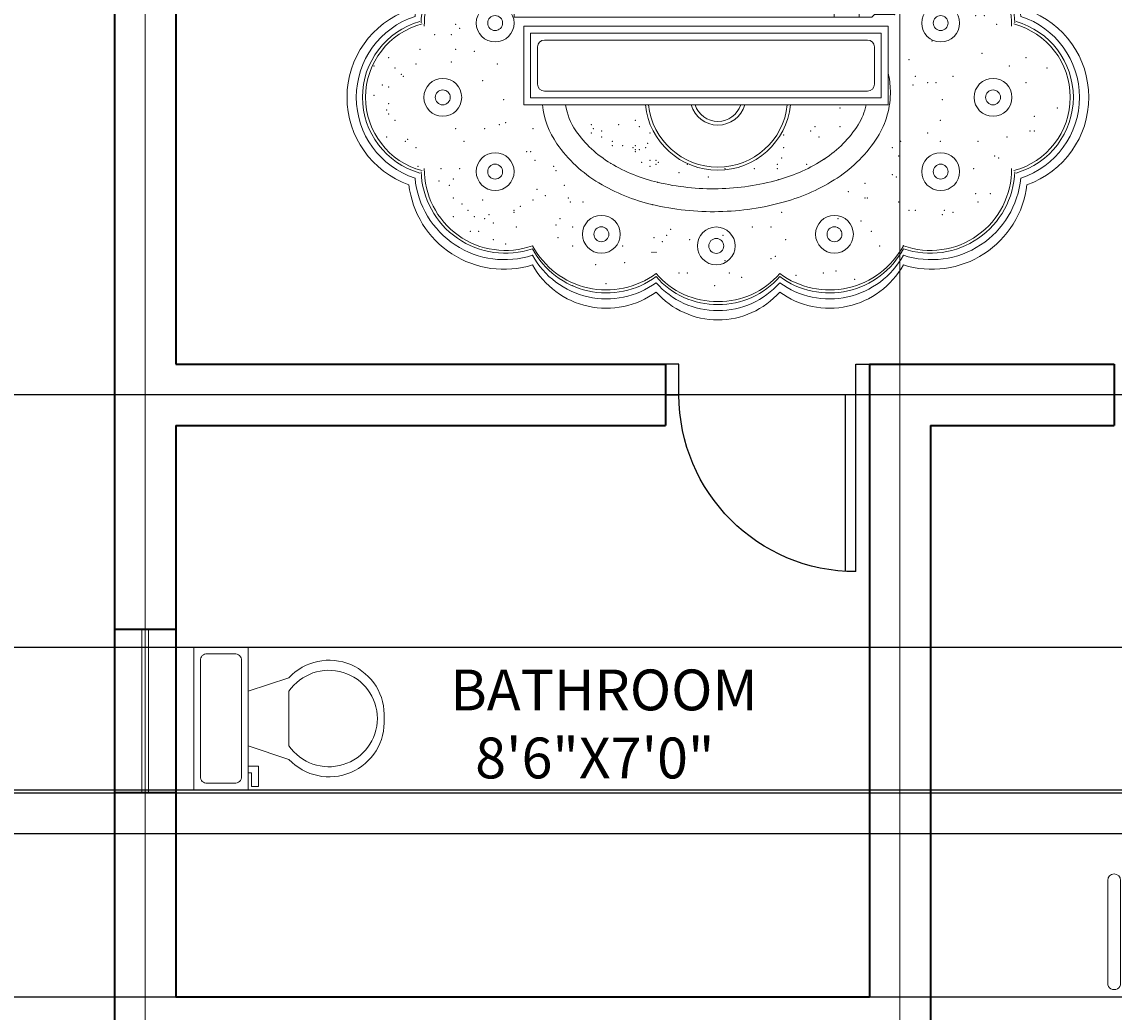
# Model space of a CAD drawing. Units: inches. Extents: x 5716 to 6907, y 12769 to 13594.
# Tile 13 of 17: x 6254 to 6414, y 13204 to 13349. Entities that reach past the tile are written whole.
import ezdxf

# ---------------------------------------------------------------- set-up
doc = ezdxf.new("R2010")
doc.units = ezdxf.units.IN
for name, color, linetype, lineweight in [('A-ANNO-DIMS', 2, 'Continuous', 18), ('A-AREA-IDEN', 7, 'Continuous', 18), ('A-DOOR', 4, 'Continuous', 25), ('A-FLOR-FIXT', 9, 'Continuous', 18), ('A-FURN', 8, 'Continuous', 18), ('A-GLAZ', 4, 'Continuous', 18), ('A-GRID', 8, 'Continuous', 13), ('A-WALL', 7, 'Continuous', 35)]:
    doc.layers.add(name, color=color, linetype=linetype, lineweight=lineweight)
doc.styles.get("Standard").update_dxf_attribs({"font": 'arial.ttf'})
doc.dimstyles.get("Standard").update_dxf_attribs({"dimtxt": 0.18, "dimasz": 0.18, "dimexe": 0.18, "dimexo": 0.0625, "dimgap": 0.09, "dimtad": 0, "dimtih": 1, "dimtoh": 1, "dimdec": 4, "dimzin": 0, "dimdsep": 46, "dimtxsty": 'Standard', "dimcen": 0.09, "dimadec": 0, "dimazin": 0, "dimtfac": 1, "dimtdec": 4, "dimtofl": 0, "dimtmove": 0, "dimatfit": 3, "dimfxl": 1, "dimtolj": 1, "dimtzin": 0, "dimarcsym": 0})

# ---------------------------------------------------------------- blocks, each defined once
blk = doc.blocks.new('A$C1EC128A1')
for p, q in [((0.1147, 3.56), (3.0187, 3.56)), ((0.1147, 3.555), (0.1147, 3.511)), ((3.0187, 3.555), (3.0187, 3.511)), ((0.1147, 3.511), (3.0187, 3.511)), ((0.2027, 3.511), (0.2027, 3.4616)), ((0.6977, 3.511), (0.6977, 3.016)), ((0.7417, 3.511), (0.7417, 2.972)), ((0.7857, 3.4835), (1.5392, 3.4835)), ((0.7857, 3.4835), (0.7857, 3.126)), ((1.5392, 3.126), (1.5392, 3.4835)), ((1.5942, 3.126), (1.5942, 3.4835)), ((1.5942, 3.4835), (2.3477, 3.4835)), ((2.3477, 3.4835), (2.3477, 3.126)), ((2.3917, 3.511), (2.3917, 3.1535)), ((2.4357, 3.511), (2.4357, 3.016)), ((2.9307, 3.511), (2.9307, 3.016)), ((0.2027, 3.4601), (0.2027, 3.016)), ((0.3741, 3.1815), (0.5297, 3.337)), ((0.3741, 3.337), (0.5297, 3.1815)), ((2.6038, 3.337), (2.7594, 3.1815)), ((2.7594, 3.337), (2.6038, 3.1815)), ((1.5392, 3.1535), (1.5942, 3.1535)), ((2.3477, 3.1535), (2.4027, 3.1535)), ((2.4027, 3.1535), (2.4027, 1.432)), ((0.7307, 2.961), (0.8957, 3.126)), ((0.7857, 3.126), (1.5392, 3.126)), ((0.9507, 3.126), (0.9507, 2.9335)), ((1.0607, 3.126), (1.0607, 2.8235)), ((1.5942, 3.126), (2.3477, 3.126)), ((0.2027, 3.016), (0.6977, 3.016)), ((1.0607, 3.0435), (2.4027, 3.0435)), ((2.9307, 3.016), (2.4357, 3.016)), ((0.7307, 2.961), (0.7307, 1.322)), ((0.7307, 2.9335), (0.9507, 2.9335)), ((0.7307, 2.8235), (1.0607, 2.8235)), ((2.1277, 1.597), (2.4027, 1.597)), ((2.1277, 1.597), (2.1277, 1.322)), ((2.2377, 1.487), (2.2377, 1.322)), ((2.2377, 1.487), (2.4027, 1.487)), ((2.2927, 1.322), (2.4027, 1.432)), ((2.3917, 1.421), (2.3917, 1.333)), ((0.7307, 1.322), (2.2927, 1.322)), ((2.3037, 1.333), (2.3917, 1.333)), ((0.7721, 1.282), (2.3633, 1.282)), ((0.7721, 0.939), (0.7721, 1.282)), ((0.8021, 1.252), (2.3333, 1.252)), ((0.8021, 0.969), (0.8021, 1.252)), ((2.3333, 1.252), (2.3333, 0.969)), ((2.3633, 1.282), (2.3633, 0.939)), ((0.8621, 1.222), (2.2733, 1.222)), ((0.8321, 1.029), (0.8321, 1.192)), ((2.3033, 1.192), (2.3033, 1.029)), ((2.3333, 0.969), (0.8021, 0.969)), ((2.2733, 0.999), (0.8621, 0.999)), ((2.3633, 0.939), (0.7721, 0.939))]:
    blk.add_line(p, q)
for centre, radius in [((0.4519, 3.2593), 0.22), ((2.6816, 3.2593), 0.22), ((0.4519, 3.2593), 0.11), ((2.6816, 3.2593), 0.11), ((0.647, 1.2961), 0.0826), ((2.593, 1.2961), 0.0826), ((0.647, 1.2961), 0.0326), ((2.593, 1.2961), 0.0326), ((0.4183, 0.9718), 0.0826), ((2.8217, 0.9718), 0.0826), ((0.4183, 0.9718), 0.0326), ((2.8217, 0.9718), 0.0326), ((0.647, 0.6475), 0.0826), ((2.593, 0.6475), 0.0826), ((0.647, 0.6475), 0.0326), ((2.593, 0.6475), 0.0326), ((1.1109, 0.3741), 0.0826), ((2.1291, 0.3741), 0.0826), ((1.1109, 0.3741), 0.0326), ((1.6128, 0.3232), 0.0826), ((2.1291, 0.3741), 0.0326), ((1.6128, 0.3232), 0.0326)]:
    blk.add_circle(centre, radius)
for centre, radius, start, end in [((0.6854, 1.3045), 0.4183, 83.7824, 173.2515), ((2.5546, 1.3045), 0.4183, 6.7485, 111.2795), ((0.6884, 1.2877), 0.3932, 83.8157, 174.53), ((2.5516, 1.2877), 0.3932, 5.47, 112.249), ((0.6921, 1.2838), 0.369, 83.9971, 177.9976), ((0.6913, 1.2866), 0.3539, 83.6051, 180.6699), ((2.5479, 1.2838), 0.369, 2.0024, 113.1536), ((2.5487, 1.2866), 0.3539, 359.3301, 114.3551), ((0.4048, 0.972), 0.4048, 109.4527, 180), ((2.8352, 0.972), 0.4048, 0, 70.5473), ((0.4119, 0.972), 0.3714, 108.0256, 180), ((0.411, 0.972), 0.3435, 105.7891, 180), ((0.4122, 0.972), 0.3312, 104.766, 180), ((2.8278, 0.972), 0.3312, 0, 75.234), ((2.829, 0.972), 0.3435, 0, 74.2109), ((2.8281, 0.972), 0.3714, 0, 71.9744), ((0.8621, 1.192), 0.03, 90, 180), ((2.2733, 1.192), 0.03, 0, 90), ((2.0084, 0.9935), 0.365, 1.1782, 13.4812), ((0.8621, 1.029), 0.03, 180, 270), ((2.2733, 1.029), 0.03, 270, 0), ((0.4048, 0.972), 0.4048, 180, 250.5473), ((0.4119, 0.972), 0.3714, 180, 251.9744), ((0.411, 0.972), 0.3435, 180, 254.2109), ((0.4122, 0.972), 0.3312, 180, 255.234), ((2.0084, 0.9935), 0.365, 327.6239, 1.1782), ((2.8278, 0.972), 0.3312, 284.766, 0), ((2.829, 0.972), 0.3435, 285.7891, 0), ((2.8281, 0.972), 0.3714, 288.0256, 0), ((2.8352, 0.972), 0.4048, 289.4527, 0), ((1.2169, 0.9773), 0.365, 186.0197, 214.7326), ((1.2169, 0.9773), 0.265, 188.3055, 214.7326), ((1.62, 0.972), 0.3185, 185.9507, 354.0493), ((1.62, 0.972), 0.305, 186.2151, 353.7849), ((1.62, 0.972), 0.1215, 195.7695, 344.2305), ((1.62, 0.972), 0.105, 198.3291, 341.6709), ((2.0084, 0.9935), 0.265, 327.6239, 348.1186), ((1.4035, 1.1066), 0.492, 214.7326, 239.1926), ((1.8167, 1.1151), 0.492, 303.1639, 327.6239), ((1.4035, 1.1066), 0.592, 214.7326, 239.1926), ((1.8167, 1.1151), 0.592, 303.1639, 327.6239), ((1.5241, 1.3089), 0.7275, 239.1926, 256.6746), ((1.6878, 1.3123), 0.7275, 285.6819, 303.1639), ((0.6921, 0.6602), 0.369, 182.0024, 288.623), ((0.6913, 0.6574), 0.3539, 179.3301, 289.5945), ((2.5487, 0.6574), 0.3539, 250.4055, 0.6699), ((2.5479, 0.6602), 0.369, 251.377, 357.9976), ((0.6854, 0.6395), 0.4183, 186.7485, 287.3233), ((0.6884, 0.6563), 0.3932, 185.47, 288.0175), ((1.5241, 1.3089), 0.8275, 239.1926, 256.6746), ((1.5995, 1.627), 1.0544, 256.6746, 271.1782), ((1.5995, 1.627), 1.0544, 271.1782, 285.6819), ((1.6878, 1.3123), 0.8275, 285.6819, 303.1639), ((2.5516, 0.6563), 0.3932, 251.9825, 354.53), ((2.5546, 0.6395), 0.4183, 252.6767, 353.2515), ((1.5995, 1.627), 1.1544, 256.6746, 271.1782), ((1.5995, 1.627), 1.1544, 271.1782, 285.6819), ((1.1328, 0.4977), 0.3665, 208.2914, 306.3479), ((1.1328, 0.4842), 0.3665, 208.2914, 306.3479), ((2.1072, 0.4977), 0.3665, 233.6521, 331.7086), ((2.1072, 0.4842), 0.3665, 233.6521, 331.7086), ((1.133, 0.4609), 0.369, 208.9302, 306.0262), ((1.1324, 0.4204), 0.3694, 209.2201, 306.079), ((2.107, 0.4609), 0.369, 233.9738, 331.0698), ((2.1076, 0.4204), 0.3694, 233.921, 330.7799), ((1.6145, 0.4295), 0.3486, 220.6393, 270.9052), ((1.6255, 0.4295), 0.3486, 269.0948, 319.3607), ((1.6145, 0.416), 0.3486, 220.6393, 270.9052), ((1.62, 0.4004), 0.3599, 221.3878, 270), ((1.6255, 0.416), 0.3486, 269.0948, 319.3607), ((1.62, 0.4004), 0.3599, 270, 318.6122), ((1.62, 0.36), 0.36, 221.4185, 270), ((1.62, 0.36), 0.36, 270, 318.5815)]:
    blk.add_arc(centre, radius, start, end)
for p in [(0.5654, 1.5652), (0.6657, 1.5561), (2.4819, 1.5378), (2.5184, 1.5744), (2.5366, 1.5378), (2.6097, 1.5378), (2.71, 1.5561), (0.4376, 1.5104), (0.5471, 1.5013), (0.5471, 1.4922), (0.6475, 1.5013), (0.465, 1.4739), (2.6735, 1.4739), (2.6735, 1.4556), (2.7648, 1.4465), (0.4285, 1.4282), (0.4285, 1.3917), (0.5562, 1.3917), (0.5927, 1.3917), (0.6566, 1.41), (2.6005, 1.4191), (2.8013, 1.4191), (0.4011, 1.3552), (0.4285, 1.3734), (2.7648, 1.346), (0.4741, 1.2912), (2.3917, 1.333), (2.7465, 1.3278), (2.7831, 1.3278), (2.8378, 1.2912), (0.3828, 1.2456), (0.4558, 1.2456), (0.4923, 1.273), (2.5549, 1.2182), (0.1821, 1.1451), (0.3189, 1.1816), (0.4741, 1.1816), (0.5562, 1.1725), (2.7739, 1.1634), (2.9656, 1.1451), (0.1182, 1.1085), (0.2094, 1.0994), (0.3007, 1.1177), (0.4558, 1.1268), (0.6566, 1.1177), (2.4545, 1.1359), (2.8926, 1.1085), (3.0568, 1.0994), (0.2368, 1.072), (0.2459, 1.0629), (2.4819, 1.0629), (2.6462, 1.0629), (0.1547, 1.0263), (0.1821, 1.0172), (0.5927, 1.0446), (2.4728, 1.0263), (2.5366, 1.0355), (2.5731, 1.0355), (2.9656, 1.0355), (0.1182, 0.9807), (0.684, 0.9624), (2.6005, 0.9624), (0.1729, 0.9167), (0.1821, 0.9441), (1.3032, 0.939), (1.3168, 0.939), (2.1533, 0.9259), (3.1025, 0.9259), (0.1821, 0.8985), (0.2094, 0.8711), (0.6931, 0.8619), (1.259, 0.8711), (2.5914, 0.8711), (3.0021, 0.8893), (0.4741, 0.8345), (0.6019, 0.8345), (0.6657, 0.8528), (0.8118, 0.8345), (0.9992, 0.8263), (1.0673, 0.8528), (1.0673, 0.8163), (1.0764, 0.8345), (1.1129, 0.8254), (1.1859, 0.8528), (1.2772, 0.8437), (1.3228, 0.8163), (2.0256, 0.8254), (2.0438, 0.8437), (2.0438, 0.8437), (2.1533, 0.8437), (2.5366, 0.8163), (2.9838, 0.8254), (3.0021, 0.8254), (0.1729, 0.798), (0.2551, 0.7797), (0.2642, 0.7889), (0.5106, 0.7797), (1.1129, 0.798), (1.1586, 0.7797), (1.3137, 0.7706), (1.9069, 0.8071), (2.0621, 0.798), (2.418, 0.7797), (2.5914, 0.7797), (2.7557, 0.7797), (2.8834, 0.798), (0.3007, 0.7523), (0.7844, 0.7341), (0.8026, 0.7341), (1.1586, 0.7615), (1.2042, 0.7615), (1.2498, 0.7523), (1.259, 0.7615), (1.259, 0.7432), (1.259, 0.7341), (1.2772, 0.7432), (1.3046, 0.7523), (1.9069, 0.7523), (2.3815, 0.7523), (2.4089, 0.7158), (2.8287, 0.7158), (0.3098, 0.6701), (0.8209, 0.6975), (0.903, 0.6701), (1.1515, 0.684), (1.1515, 0.684), (1.1515, 0.684), (1.2863, 0.6884), (1.3228, 0.6975), (1.3228, 0.6701), (1.3502, 0.6975), (1.3502, 0.6793), (1.3593, 0.6884), (1.4871, 0.6793), (1.8795, 0.6793), (1.8978, 0.7067), (2.0073, 0.6793), (2.0858, 0.7033), (2.8469, 0.7067), (0.4102, 0.661), (0.4923, 0.661), (0.9122, 0.6519), (1.4506, 0.6427), (1.5784, 0.6245), (1.6514, 0.661), (1.6514, 0.661), (1.7792, 0.661), (1.8795, 0.661), (2.3815, 0.6336), (2.3997, 0.6245), (2.7374, 0.661), (0.4011, 0.6062), (0.4467, 0.5879), (0.465, 0.6153), (0.9487, 0.5879), (1.3564, 0.601), (1.8845, 0.6118), (2.2629, 0.597), (0.465, 0.5331), (0.83, 0.5696), (0.8665, 0.5422), (0.9669, 0.5331), (2.1898, 0.5605), (2.2629, 0.5331), (2.272, 0.5331), (2.7465, 0.5514), (2.8104, 0.5514), (0.5015, 0.5057), (0.5289, 0.4783), (0.5927, 0.524), (0.7296, 0.4783), (0.757, 0.4966), (0.8118, 0.524), (0.976, 0.5148), (1.0308, 0.5148), (1.3334, 0.5037), (2.4089, 0.5148), (2.4545, 0.4783), (2.4819, 0.4783), (2.6097, 0.4783), (2.7557, 0.5148), (0.465, 0.4509), (0.5562, 0.4509), (0.6019, 0.4418), (0.6201, 0.46), (0.7296, 0.4692), (0.9304, 0.4418), (1.8978, 0.4692), (2.1442, 0.4418), (2.2446, 0.4326), (2.6005, 0.46), (2.6462, 0.4692), (0.538, 0.387), (0.5745, 0.387), (0.6384, 0.4235), (0.7388, 0.4052), (0.7388, 0.4052), (0.9122, 0.4144), (0.9852, 0.4052), (1.4141, 0.3961), (1.77, 0.4052), (1.8522, 0.4052), (2.2902, 0.387), (0.6384, 0.3504), (0.9213, 0.3596), (1.3411, 0.3596), (1.3776, 0.3413), (1.3959, 0.3687), (1.4962, 0.3504), (1.6423, 0.3687), (1.9161, 0.3504), (0.6931, 0.3322), (0.9852, 0.323), (1.2042, 0.323), (1.332, 0.2956), (1.3411, 0.2956), (1.3502, 0.2956), (2.3267, 0.323), (2.43, 0.324), (0.81, 0.2824), (1.0856, 0.2408), (1.2133, 0.25), (1.6514, 0.2591), (1.8522, 0.2682), (1.8704, 0.2774), (1.35, 0.2025), (1.4506, 0.2043), (1.4871, 0.2043), (1.6696, 0.2043), (1.9617, 0.1952), (2.0803, 0.2043), (2.1351, 0.2134), (0.9852, 0.1495), (1.1312, 0.1586), (1.6058, 0.1495), (1.7244, 0.186), (2.2172, 0.1769)]:
    blk.add_point(p)
blk = doc.blocks.new('A$C405465A0')
for p, q in [((1.1305, 2.1034), (1.5301, 2.1034)), ((1.5301, 2.0534), (1.1305, 2.0534)), ((1.1304, 1.6481), (1.1055, 2.0017)), ((1.279, 2.0284), (1.1105, 1.9312)), ((1.4665, 2.0284), (1.1178, 1.8271)), ((1.1305, 2.0284), (1.5301, 2.0284)), ((1.1428, 1.625), (1.1428, 2.0284)), ((1.5427, 1.8271), (1.1941, 2.0284)), ((1.2365, 1.625), (1.2365, 2.0284)), ((1.3303, 1.625), (1.3303, 2.0284)), ((1.5501, 1.9312), (1.3816, 2.0284)), ((1.424, 1.625), (1.424, 2.0284)), ((1.5178, 1.625), (1.5178, 2.0284)), ((1.555, 2.0017), (1.5301, 1.6481)), ((1.5354, 1.7231), (1.1078, 1.97)), ((1.5528, 1.97), (1.1252, 1.7231)), ((0.9452, 1.8803), (0.5455, 1.8803)), ((2.1342, 1.8803), (1.7345, 1.8803)), ((0.5455, 1.8303), (0.9452, 1.8303)), ((1.5178, 1.625), (1.1157, 1.8572)), ((1.5449, 1.8572), (1.1428, 1.625)), ((1.7345, 1.8303), (2.1342, 1.8303)), ((0.5268, 1.6904), (0.7259, 1.8053)), ((0.9452, 1.8053), (0.5455, 1.8053)), ((0.5578, 1.6), (0.5578, 1.8053)), ((0.5578, 1.6), (0.9134, 1.8053)), ((0.5773, 1.8053), (0.9328, 1.6)), ((0.6516, 1.6), (0.6516, 1.8053)), ((0.7453, 1.6), (0.7453, 1.8053)), ((0.7648, 1.8053), (0.9639, 1.6904)), ((0.8391, 1.6), (0.8391, 1.8053)), ((0.9328, 1.6), (0.9328, 1.8053)), ((1.7158, 1.6904), (1.9149, 1.8053)), ((2.1342, 1.8053), (1.7345, 1.8053)), ((1.7468, 1.6), (1.7468, 1.8053)), ((1.7468, 1.6), (2.1024, 1.8053)), ((1.7663, 1.8053), (2.1218, 1.6)), ((1.8406, 1.6), (1.8406, 1.8053)), ((1.9343, 1.6), (1.9343, 1.8053)), ((1.9538, 1.8053), (2.1529, 1.6904)), ((2.0281, 1.6), (2.0281, 1.8053)), ((2.1218, 1.6), (2.1218, 1.8053)), ((0.5206, 1.7786), (0.5332, 1.6)), ((0.9575, 1.6), (0.9701, 1.7786)), ((1.3303, 1.625), (1.1237, 1.7443)), ((1.5369, 1.7443), (1.3303, 1.625)), ((1.7096, 1.7786), (1.7222, 1.6)), ((2.1465, 1.6), (2.1591, 1.7786)), ((0.5242, 1.7277), (0.7453, 1.6)), ((0.7453, 1.6), (0.9665, 1.7277)), ((1.7132, 1.7277), (1.9343, 1.6)), ((1.9343, 1.6), (2.1555, 1.7277)), ((1.1428, 1.625), (1.1316, 1.6315)), ((1.5052, 1.625), (1.1554, 1.625)), ((1.529, 1.6315), (1.5178, 1.625)), ((2.3803, 1.6), (0.2803, 1.6)), ((0.2803, 1.6), (0.2803, 0.5)), ((0.4356, 1.5842), (0.3956, 1.553)), ((0.5827, 1.5379), (0.4356, 1.5842)), ((0.5321, 1.6149), (0.5578, 1.6)), ((0.5332, 1.6), (0.9575, 1.6)), ((0.7152, 1.6), (0.7236, 1.5766)), ((0.7236, 1.5766), (0.7578, 1.4998)), ((0.9055, 1.5469), (0.8836, 1.6)), ((0.9328, 1.6), (0.9586, 1.6149)), ((1.0212, 1.6), (1.0194, 1.5656)), ((1.1269, 1.5706), (1.1432, 1.6)), ((1.1922, 1.5507), (1.214, 1.6)), ((1.3907, 1.6), (1.3616, 1.5541)), ((1.7211, 1.6149), (1.7468, 1.6)), ((1.7222, 1.6), (2.1465, 1.6)), ((1.9093, 1.5754), (1.8386, 1.5427)), ((1.9386, 1.6), (1.9093, 1.5754)), ((2.1086, 1.5664), (2.17, 1.6)), ((2.1218, 1.6), (2.1476, 1.6149)), ((2.3803, 1.5967), (2.3153, 1.558)), ((2.3803, 0.5), (2.3803, 1.6)), ((0.3956, 1.553), (0.3856, 1.5163)), ((0.4482, 1.5094), (0.4582, 1.5336)), ((0.4582, 1.5336), (0.5016, 1.5339)), ((0.5016, 1.5339), (0.54, 1.5204)), ((0.6365, 1.5019), (0.5827, 1.5379)), ((0.9296, 1.4669), (0.9055, 1.5469)), ((1.0194, 1.5656), (1.026, 1.5003)), ((1.1178, 1.5243), (1.1269, 1.5706)), ((1.1887, 1.5196), (1.1922, 1.5507)), ((1.3616, 1.5541), (1.3027, 1.5125)), ((1.7679, 1.5301), (1.6627, 1.5271)), ((1.8386, 1.5427), (1.7679, 1.5301)), ((1.9962, 1.5248), (2.1086, 1.5664)), ((2.3153, 1.558), (2.1962, 1.4994)), ((0.3856, 1.5163), (0.4538, 1.4363)), ((0.4595, 1.4847), (0.4482, 1.5094)), ((0.54, 1.5204), (0.5786, 1.5)), ((0.5786, 1.5), (0.6151, 1.4744)), ((0.7193, 1.4377), (0.6365, 1.5019)), ((0.7578, 1.4998), (0.7752, 1.4525)), ((1.026, 1.5003), (1.0343, 1.4559)), ((1.1128, 1.4699), (1.1178, 1.5243)), ((1.2089, 1.4946), (1.1887, 1.5196)), ((1.2618, 1.4976), (1.2089, 1.4946)), ((1.3027, 1.5125), (1.2618, 1.4976)), ((1.446, 1.5079), (1.3392, 1.4609)), ((1.5543, 1.5261), (1.446, 1.5079)), ((1.6627, 1.5271), (1.5543, 1.5261)), ((1.717, 1.474), (1.8488, 1.4892)), ((1.8488, 1.4892), (1.9962, 1.5248)), ((2.1962, 1.4994), (2.0887, 1.4564)), ((2.215, 1.4381), (2.3447, 1.5068)), ((2.3447, 1.5068), (2.3803, 1.5269)), ((0.3744, 1.3943), (0.2803, 1.458)), ((0.4876, 1.4521), (0.4595, 1.4847)), ((0.5099, 1.4328), (0.4876, 1.4521)), ((0.6151, 1.4744), (0.6557, 1.4351)), ((0.7752, 1.4525), (0.7871, 1.4053)), ((0.9436, 1.385), (0.9296, 1.4669)), ((1.0343, 1.4559), (1.0488, 1.3883)), ((1.1133, 1.4295), (1.1128, 1.4699)), ((1.3392, 1.4609), (1.2655, 1.4131)), ((1.4396, 1.445), (1.5179, 1.4625)), ((1.5179, 1.4625), (1.717, 1.474)), ((2.0887, 1.4564), (1.9879, 1.4268)), ((0.4538, 1.4363), (0.5034, 1.394)), ((0.5366, 1.4137), (0.5099, 1.4328)), ((0.5694, 1.3947), (0.5366, 1.4137)), ((0.6557, 1.4351), (0.6746, 1.4025)), ((0.6746, 1.4025), (0.674, 1.3825)), ((0.7442, 1.4091), (0.7193, 1.4377)), ((0.746, 1.3555), (0.7442, 1.4091)), ((0.7871, 1.4053), (0.7898, 1.3706)), ((1.1222, 1.3821), (1.1133, 1.4295)), ((1.2655, 1.4131), (1.2034, 1.3712)), ((1.3398, 1.3841), (1.4396, 1.445)), ((1.9879, 1.4268), (1.8502, 1.4019)), ((2.1089, 1.3912), (2.215, 1.4381)), ((0.4543, 1.3479), (0.3744, 1.3943)), ((0.5034, 1.394), (0.551, 1.3648)), ((0.551, 1.3648), (0.5952, 1.3458)), ((0.597, 1.3823), (0.5694, 1.3947)), ((0.6281, 1.3731), (0.597, 1.3823)), ((0.654, 1.3714), (0.6281, 1.3731)), ((0.674, 1.3825), (0.654, 1.3714)), ((0.7898, 1.3706), (0.7722, 1.3216)), ((0.9447, 1.3133), (0.9436, 1.385)), ((1.0488, 1.3883), (1.0626, 1.2943)), ((1.1508, 1.3537), (1.1222, 1.3821)), ((1.2034, 1.3712), (1.1508, 1.3537)), ((1.2659, 1.3078), (1.3398, 1.3841)), ((1.4616, 1.3726), (1.4211, 1.3426)), ((1.5407, 1.3902), (1.4616, 1.3726)), ((1.6315, 1.3907), (1.5407, 1.3902)), ((1.7291, 1.3922), (1.6315, 1.3907)), ((1.8502, 1.4019), (1.7291, 1.3922)), ((1.8869, 1.3472), (1.9689, 1.3731)), ((1.9689, 1.3731), (2.0551, 1.3789)), ((2.0551, 1.3789), (2.1089, 1.3912)), ((2.1327, 1.3477), (2.1998, 1.3905)), ((2.1998, 1.3905), (2.271, 1.4021)), ((2.271, 1.4021), (2.3264, 1.3943)), ((2.3264, 1.3943), (2.3803, 1.3943)), ((0.2803, 1.3424), (0.3226, 1.3046)), ((0.523, 1.3203), (0.4543, 1.3479)), ((0.6007, 1.301), (0.523, 1.3203)), ((0.5952, 1.3458), (0.6524, 1.335)), ((0.6524, 1.335), (0.7159, 1.3352)), ((0.7159, 1.3352), (0.746, 1.3555)), ((0.7722, 1.3216), (0.7385, 1.3018)), ((1.4211, 1.3426), (1.398, 1.3071)), ((1.8267, 1.2783), (1.8309, 1.3257)), ((1.8309, 1.3257), (1.8869, 1.3472)), ((2.1112, 1.3052), (2.1327, 1.3477)), ((2.2336, 1.2914), (2.2346, 1.3391)), ((2.2346, 1.3391), (2.2726, 1.3593)), ((2.2726, 1.3593), (2.339, 1.3581)), ((2.339, 1.3581), (2.3803, 1.3581)), ((0.3797, 1.2052), (0.2803, 1.2816)), ((0.3226, 1.3046), (0.3891, 1.2586)), ((0.6623, 1.3018), (0.6007, 1.301)), ((0.7385, 1.3018), (0.6623, 1.3018)), ((0.9305, 1.2479), (0.9447, 1.3133)), ((1.0626, 1.2943), (1.06, 1.2384)), ((1.1689, 1.1968), (1.2659, 1.3078)), ((1.398, 1.3071), (1.412, 1.2681)), ((1.8814, 1.2462), (1.8267, 1.2783)), ((2.1264, 1.2714), (2.1112, 1.3052)), ((2.2746, 1.2504), (2.2336, 1.2914)), ((0, 1.2499), (0, 0.8502)), ((0.05, 0.8502), (0.05, 1.2499)), ((0.075, 1.0695), (0.19, 1.2686)), ((0.075, 1.2499), (0.075, 0.8502)), ((0.2803, 1.2375), (0.075, 1.2375)), ((0.075, 0.882), (0.2803, 1.2375)), ((0.2803, 1.2622), (0.1018, 1.2748)), ((0.2803, 1.05), (0.1526, 1.2712)), ((0.2803, 1.2375), (0.2654, 1.2633)), ((0.2803, 0.8379), (0.2803, 1.2622)), ((0.2803, 1.2498), (0.478, 1.1251)), ((0.3891, 1.2586), (0.4808, 1.2074)), ((0.8894, 1.1911), (0.9305, 1.2479)), ((1.06, 1.2384), (1.0402, 1.1815)), ((1.412, 1.2681), (1.4535, 1.2416)), ((1.4535, 1.2416), (1.5203, 1.2085)), ((1.9819, 1.2225), (1.8814, 1.2462)), ((2.171, 1.2386), (2.1264, 1.2714)), ((2.2593, 1.2028), (2.171, 1.2386)), ((2.3417, 1.2285), (2.2746, 1.2504)), ((2.3803, 1.2622), (2.5588, 1.2748)), ((2.3803, 1.05), (2.508, 1.2712)), ((2.3803, 1.2375), (2.3951, 1.2633)), ((2.3803, 0.8379), (2.3803, 1.2622)), ((2.3803, 1.2375), (2.5856, 1.2375)), ((2.5856, 0.882), (2.3803, 1.2375)), ((2.5856, 1.0695), (2.4706, 1.2686)), ((2.5856, 1.2499), (2.5856, 0.8502)), ((2.6106, 0.8502), (2.6106, 1.2499)), ((2.6606, 1.2499), (2.6606, 0.8502)), ((0.2803, 0.8625), (0.075, 1.2181)), ((0.3728, 1.1548), (0.2803, 1.2123)), ((0.4682, 1.1454), (0.3797, 1.2052)), ((0.4808, 1.2074), (0.5771, 1.1712)), ((0.8213, 1.159), (0.8894, 1.1911)), ((1.0809, 1.1136), (1.1689, 1.1968)), ((1.5203, 1.2085), (1.5912, 1.2143)), ((1.5912, 1.2143), (1.7027, 1.2151)), ((1.7027, 1.2151), (1.8282, 1.1987)), ((1.8282, 1.1987), (1.9236, 1.1792)), ((2.1048, 1.2108), (1.9819, 1.2225)), ((2.1888, 1.194), (2.1048, 1.2108)), ((2.2653, 1.1704), (2.1888, 1.194)), ((2.3339, 1.1841), (2.2593, 1.2028)), ((2.3803, 1.226), (2.3417, 1.2285)), ((2.3803, 0.8625), (2.5856, 1.2181)), ((0.4405, 1.1078), (0.3728, 1.1548)), ((0.5771, 1.1712), (0.7161, 1.1491)), ((0.7161, 1.1491), (0.8213, 1.159)), ((1.0402, 1.1815), (0.9932, 1.1252)), ((1.4537, 1.1662), (1.3237, 1.1316)), ((1.6097, 1.1755), (1.4537, 1.1662)), ((1.757, 1.1624), (1.6097, 1.1755)), ((1.9184, 1.131), (1.757, 1.1624)), ((1.9236, 1.1792), (2.049, 1.1552)), ((2.049, 1.1552), (2.1515, 1.1303)), ((2.3396, 1.1432), (2.2653, 1.1704)), ((2.3803, 1.1754), (2.3339, 1.1841)), ((0.2803, 1.1438), (0.075, 1.1438)), ((0.2803, 1.1471), (0.3609, 1.0879)), ((0.5402, 1.0464), (0.4405, 1.1078)), ((0.5225, 1.114), (0.4682, 1.1454)), ((0.478, 1.1251), (0.576, 1.067)), ((0.5954, 1.0801), (0.5225, 1.114)), ((0.9932, 1.1252), (0.9121, 1.0739)), ((0.9908, 1.0561), (1.0809, 1.1136)), ((1.3237, 1.1316), (1.2549, 1.1012)), ((1.4887, 1.0901), (1.6473, 1.1088)), ((1.6473, 1.1088), (1.7544, 1.0961)), ((2.0769, 1.0887), (1.9184, 1.131)), ((2.1515, 1.1303), (2.2486, 1.0908)), ((2.3803, 1.126), (2.3396, 1.1432)), ((2.3803, 1.1438), (2.5856, 1.1438)), ((0.3609, 1.0879), (0.5015, 1.0099)), ((0.576, 1.067), (0.7146, 1.0163)), ((0.6603, 1.0585), (0.5954, 1.0801)), ((0.9121, 1.0739), (0.863, 1.056)), ((1.2549, 1.1012), (1.1432, 1.0368)), ((1.3755, 1.0479), (1.4887, 1.0901)), ((1.7544, 1.0961), (1.9207, 1.0564)), ((2.2686, 1.0282), (2.0769, 1.0887)), ((2.2486, 1.0908), (2.3803, 1.048)), ((0.2803, 1.05), (0.075, 1.05)), ((0.19, 0.8315), (0.075, 1.0306)), ((0.1526, 0.8289), (0.2803, 1.05)), ((0.3078, 1.029), (0.2803, 1.0458)), ((0.346, 1.0052), (0.3078, 1.029)), ((0.6261, 1.0028), (0.5402, 1.0464)), ((0.7308, 1.0454), (0.6603, 1.0585)), ((0.7897, 1.0439), (0.7308, 1.0454)), ((0.863, 1.056), (0.7897, 1.0439)), ((0.7979, 1.0084), (0.9069, 1.0237)), ((0.9069, 1.0237), (0.9908, 1.0561)), ((1.1432, 1.0368), (1.0559, 0.9876)), ((1.2543, 0.9907), (1.3755, 1.0479)), ((1.9207, 1.0564), (2.1244, 0.9922)), ((2.3803, 0.9983), (2.2686, 1.0282)), ((2.3803, 1.05), (2.5856, 1.05)), ((2.508, 0.8289), (2.3803, 1.05)), ((2.4706, 0.8315), (2.5856, 1.0306)), ((0.4051, 0.9771), (0.346, 1.0052)), ((0.5015, 1.0099), (0.6086, 0.961)), ((0.7415, 0.9604), (0.6261, 1.0028)), ((0.7146, 1.0163), (0.7979, 1.0084)), ((1.0559, 0.9876), (0.958, 0.9508)), ((1.1244, 0.9348), (1.2543, 0.9907)), ((2.1244, 0.9922), (2.2495, 0.9522)), ((0.2803, 0.9563), (0.075, 0.9563)), ((0.4579, 0.9575), (0.4051, 0.9771)), ((0.5195, 0.9378), (0.4579, 0.9575)), ((0.5818, 0.918), (0.5195, 0.9378)), ((0.6086, 0.961), (0.7339, 0.9201)), ((0.8579, 0.9417), (0.7415, 0.9604)), ((0.958, 0.9508), (0.8579, 0.9417)), ((1.4378, 0.9282), (1.5224, 0.9439)), ((1.5224, 0.9439), (1.6187, 0.9581)), ((1.6187, 0.9581), (1.7607, 0.9676)), ((1.7607, 0.9676), (1.9339, 0.9563)), ((1.9339, 0.9563), (2.0478, 0.9301)), ((2.2495, 0.9522), (2.3803, 0.9025)), ((2.3803, 0.9563), (2.5856, 0.9563)), ((0.309, 0.9074), (0.2803, 0.9224)), ((0.342, 0.8943), (0.309, 0.9074)), ((0.3823, 0.8837), (0.342, 0.8943)), ((0.6352, 0.8954), (0.5818, 0.918)), ((0.6712, 0.8671), (0.6352, 0.8954)), ((0.7339, 0.9201), (0.8463, 0.9008)), ((0.8463, 0.9008), (0.9714, 0.9002)), ((0.9714, 0.9002), (1.1244, 0.9348)), ((1.224, 0.8829), (1.301, 0.9003)), ((1.301, 0.9003), (1.4378, 0.9282)), ((2.0478, 0.9301), (2.1209, 0.9013)), ((2.1209, 0.9013), (2.214, 0.8459)), ((0.2803, 0.8625), (0.075, 0.8625)), ((0.2654, 0.8368), (0.2803, 0.8625)), ((0.4349, 0.876), (0.3823, 0.8837)), ((0.4843, 0.8652), (0.4349, 0.876)), ((0.5229, 0.85), (0.4843, 0.8652)), ((0.6805, 0.8424), (0.6712, 0.8671)), ((0.9468, 0.8025), (1.1125, 0.8545)), ((1.1125, 0.8545), (1.224, 0.8829)), ((1.5313, 0.864), (1.3995, 0.834)), ((1.6341, 0.8806), (1.5313, 0.864)), ((1.7415, 0.8904), (1.6341, 0.8806)), ((1.8296, 0.8853), (1.7415, 0.8904)), ((1.9317, 0.8609), (1.8296, 0.8853)), ((2.0406, 0.8138), (1.9317, 0.8609)), ((2.3803, 0.8625), (2.5856, 0.8625)), ((2.3951, 0.8368), (2.3803, 0.8625)), ((0.1018, 0.8253), (0.2803, 0.8379)), ((0.5441, 0.8372), (0.5229, 0.85)), ((0.5622, 0.8164), (0.5441, 0.8372)), ((0.5634, 0.7968), (0.5622, 0.8164)), ((0.6434, 0.7666), (0.675, 0.8159)), ((0.675, 0.8159), (0.6805, 0.8424)), ((1.3995, 0.834), (1.2818, 0.7979)), ((2.1229, 0.7618), (2.0406, 0.8138)), ((2.214, 0.8459), (2.297, 0.7736)), ((2.5588, 0.8253), (2.3803, 0.8379)), ((0.5313, 0.7537), (0.5562, 0.7809)), ((0.5562, 0.7809), (0.5634, 0.7968)), ((0.603, 0.7231), (0.6434, 0.7666)), ((0.8288, 0.7556), (0.9468, 0.8025)), ((1.2818, 0.7979), (1.131, 0.7357)), ((1.4547, 0.7504), (1.6229, 0.7863)), ((1.6229, 0.7863), (1.7436, 0.7907)), ((1.7436, 0.7907), (1.8858, 0.7711)), ((1.8858, 0.7711), (1.9957, 0.7333)), ((2.297, 0.7736), (2.3432, 0.7176)), ((0.4801, 0.7185), (0.5313, 0.7537)), ((0.5568, 0.6828), (0.603, 0.7231)), ((0.6995, 0.6921), (0.8288, 0.7556)), ((1.131, 0.7357), (0.9946, 0.6604)), ((1.2995, 0.6899), (1.4547, 0.7504)), ((1.9957, 0.7333), (2.0772, 0.6873)), ((2.1698, 0.724), (2.1229, 0.7618)), ((2.2541, 0.6328), (2.1698, 0.724)), ((0.3723, 0.6742), (0.4317, 0.6944)), ((0.4317, 0.6944), (0.4801, 0.7185)), ((0.499, 0.6426), (0.5568, 0.6828)), ((0.6181, 0.6464), (0.6995, 0.6921)), ((1.2062, 0.6433), (1.2995, 0.6899)), ((1.4772, 0.6838), (1.4124, 0.6631)), ((1.554, 0.696), (1.4772, 0.6838)), ((1.6333, 0.6993), (1.554, 0.696)), ((1.7153, 0.696), (1.6333, 0.6993)), ((1.7865, 0.6892), (1.7153, 0.696)), ((1.8794, 0.6748), (1.7865, 0.6892)), ((2.0772, 0.6873), (2.1261, 0.6491)), ((2.3432, 0.7176), (2.3803, 0.6555)), ((0.2803, 0.6573), (0.312, 0.6622)), ((0.312, 0.6622), (0.3723, 0.6742)), ((0.4497, 0.615), (0.499, 0.6426)), ((0.5546, 0.6082), (0.6181, 0.6464)), ((0.9946, 0.6604), (0.8746, 0.5766)), ((1.1078, 0.5882), (1.2062, 0.6433)), ((1.4124, 0.6631), (1.3518, 0.6302)), ((1.4712, 0.6079), (1.5115, 0.6388)), ((1.5115, 0.6388), (1.5744, 0.6543)), ((1.5744, 0.6543), (1.6677, 0.668)), ((1.6031, 0.6361), (1.6918, 0.6436)), ((1.6677, 0.668), (1.7434, 0.6684)), ((1.6918, 0.6436), (1.8075, 0.6404)), ((1.7434, 0.6684), (1.8417, 0.6617)), ((1.8075, 0.6404), (1.8682, 0.6312)), ((1.8417, 0.6617), (1.8785, 0.6547)), ((1.8785, 0.6547), (1.9243, 0.6434)), ((1.9674, 0.6548), (1.8794, 0.6748)), ((1.9243, 0.6434), (1.9761, 0.6102)), ((2.0494, 0.621), (1.9674, 0.6548)), ((2.1261, 0.6491), (2.1688, 0.6067)), ((0.3813, 0.5837), (0.4497, 0.615)), ((0.4385, 0.5349), (0.5546, 0.6082)), ((1.3133, 0.5983), (1.2908, 0.5736)), ((1.3518, 0.6302), (1.3133, 0.5983)), ((1.3959, 0.5264), (1.4712, 0.6079)), ((1.4828, 0.5927), (1.5188, 0.6159)), ((1.5188, 0.6159), (1.6031, 0.6361)), ((1.5621, 0.583), (1.5815, 0.6002)), ((1.5815, 0.6002), (1.641, 0.6183)), ((1.641, 0.6183), (1.6861, 0.6235)), ((1.6861, 0.6235), (1.7353, 0.624)), ((1.7353, 0.624), (1.7765, 0.6204)), ((1.7765, 0.6204), (1.811, 0.6136)), ((1.811, 0.6136), (1.8414, 0.6025)), ((1.8414, 0.6025), (1.8603, 0.5873)), ((1.8682, 0.6312), (1.909, 0.622)), ((1.909, 0.622), (1.9497, 0.5991)), ((1.9497, 0.5991), (1.9595, 0.5705)), ((1.9761, 0.6102), (2.006, 0.5625)), ((2.1071, 0.5697), (2.0494, 0.621)), ((2.1688, 0.6067), (2.197, 0.5721)), ((2.3022, 0.5551), (2.2541, 0.6328)), ((0.2803, 0.5477), (0.3159, 0.5583)), ((0.3159, 0.5583), (0.3813, 0.5837)), ((0.8746, 0.5766), (0.8225, 0.5348)), ((1.0064, 0.5273), (1.1078, 0.5882)), ((1.2908, 0.5736), (1.2556, 0.52)), ((1.4736, 0.5658), (1.4828, 0.5927)), ((1.4775, 0.5489), (1.4736, 0.5658)), ((1.572, 0.557), (1.5621, 0.583)), ((1.5997, 0.5436), (1.572, 0.557)), ((1.8611, 0.5702), (1.8321, 0.5488)), ((1.8603, 0.5873), (1.8611, 0.5702)), ((1.9595, 0.5705), (1.9448, 0.5456)), ((2.006, 0.5625), (2.0103, 0.5395)), ((2.1338, 0.529), (2.1071, 0.5697)), ((2.197, 0.5721), (2.2242, 0.5314)), ((2.3248, 0.5), (2.3022, 0.5551)), ((0.3857, 0.5), (0.4385, 0.5349)), ((0.8225, 0.5348), (0.7878, 0.5)), ((0.9657, 0.5), (1.0064, 0.5273)), ((1.2556, 0.52), (1.2455, 0.5)), ((1.3784, 0.5), (1.3959, 0.5264)), ((1.5273, 0.534), (1.4775, 0.5489)), ((1.6327, 0.513), (1.5273, 0.534)), ((1.6329, 0.5353), (1.5997, 0.5436)), ((1.685, 0.5094), (1.6327, 0.513)), ((1.6895, 0.5294), (1.6329, 0.5353)), ((1.7388, 0.53), (1.6895, 0.5294)), ((1.7906, 0.5103), (1.7331, 0.5091)), ((1.7888, 0.5363), (1.7388, 0.53)), ((1.8321, 0.5488), (1.7888, 0.5363)), ((1.8503, 0.5169), (1.7906, 0.5103)), ((1.9108, 0.5271), (1.8503, 0.5169)), ((1.9448, 0.5456), (1.9108, 0.5271)), ((2.0103, 0.5395), (2.0069, 0.5)), ((2.1506, 0.5), (2.1338, 0.529)), ((2.2242, 0.5314), (2.2363, 0.5)), ((0.2803, 0.5), (2.3803, 0.5)), ((0.5126, 0.2463), (0.9147, 0.4784)), ((0.5205, 0.3591), (0.7272, 0.4784)), ((0.5285, 0.4719), (0.5397, 0.4784)), ((0.5397, 0.4784), (0.5397, 0.075)), ((0.5397, 0.4784), (0.9417, 0.2463)), ((0.5522, 0.4784), (0.9021, 0.4784)), ((0.6334, 0.4784), (0.6334, 0.075)), ((0.7272, 0.4784), (0.7272, 0.075)), ((0.7272, 0.4784), (0.9338, 0.3591)), ((0.8209, 0.4784), (0.8209, 0.075)), ((0.9147, 0.4784), (0.9147, 0.075)), ((0.9147, 0.4784), (0.9258, 0.4719)), ((1.1055, 0.3215), (1.1181, 0.5)), ((1.1091, 0.3724), (1.3303, 0.5)), ((1.1171, 0.4852), (1.1428, 0.5)), ((1.1181, 0.5), (1.5425, 0.5)), ((1.1428, 0.5), (1.1428, 0.2948)), ((1.1428, 0.5), (1.4984, 0.2948)), ((1.1622, 0.2948), (1.5178, 0.5)), ((1.2365, 0.5), (1.2365, 0.2948)), ((1.3303, 0.5), (1.3303, 0.2948)), ((1.3303, 0.5), (1.5515, 0.3724)), ((1.424, 0.5), (1.424, 0.2948)), ((1.5178, 0.5), (1.5178, 0.2948)), ((1.5178, 0.5), (1.5435, 0.4852)), ((1.5425, 0.5), (1.555, 0.3215)), ((1.7331, 0.5091), (1.685, 0.5094)), ((1.7096, 0.3215), (1.7222, 0.5)), ((1.7132, 0.3724), (1.9343, 0.5)), ((1.7211, 0.4852), (1.7468, 0.5)), ((1.7222, 0.5), (2.1465, 0.5)), ((1.7468, 0.5), (1.7468, 0.2948)), ((1.7468, 0.5), (2.1024, 0.2948)), ((1.7663, 0.2948), (2.1218, 0.5)), ((1.8406, 0.5), (1.8406, 0.2948)), ((1.9343, 0.5), (1.9343, 0.2948)), ((1.9343, 0.5), (2.1555, 0.3724)), ((2.0281, 0.5), (2.0281, 0.2948)), ((2.1218, 0.5), (2.1218, 0.2948)), ((2.1218, 0.5), (2.1476, 0.4852)), ((2.1465, 0.5), (2.1591, 0.3215)), ((0.5024, 0.1018), (0.5273, 0.4553)), ((0.927, 0.4553), (0.9519, 0.1018)), ((1.1118, 0.4097), (1.3109, 0.2948)), ((1.3497, 0.2948), (1.5488, 0.4097)), ((1.7158, 0.4097), (1.9149, 0.2948)), ((1.9538, 0.2948), (2.1529, 0.4097)), ((0.5046, 0.1334), (0.9323, 0.3803)), ((0.522, 0.3803), (0.9497, 0.1334)), ((0.5147, 0.2763), (0.8634, 0.075)), ((0.591, 0.075), (0.9396, 0.2763)), ((1.5301, 0.2948), (1.1305, 0.2948)), ((1.1305, 0.2698), (1.5301, 0.2698)), ((2.1342, 0.2948), (1.7345, 0.2948)), ((1.7345, 0.2698), (2.1342, 0.2698)), ((1.5301, 0.2198), (1.1305, 0.2198)), ((2.1342, 0.2198), (1.7345, 0.2198)), ((0.5074, 0.1723), (0.6759, 0.075)), ((0.7785, 0.075), (0.9469, 0.1723)), ((0.927, 0.075), (0.5273, 0.075)), ((0.5273, 0.05), (0.927, 0.05)), ((0.927, 0), (0.5273, 0))]:
    blk.add_line(p, q)
for centre, start, end in [((1.1305, 2.0784), 90, 270), ((1.5301, 2.0784), 270, 90), ((1.1305, 2.0034), 90, 184.0274), ((1.5301, 2.0034), 355.9726, 90), ((0.5455, 1.8553), 90, 270), ((0.9452, 1.8553), 270, 90), ((1.7345, 1.8553), 90, 270), ((2.1342, 1.8553), 270, 90), ((0.5455, 1.7803), 90, 184.0274), ((0.9452, 1.7803), 355.9726, 90), ((1.7345, 1.7803), 90, 184.0274), ((2.1342, 1.7803), 355.9726, 90), ((1.1554, 1.65), 184.3987, 270), ((1.5052, 1.65), 270, 355.6013), ((0.025, 1.2499), 0, 180), ((0.1, 1.2499), 85.9726, 180), ((2.5606, 1.2499), 0, 94.0274), ((2.6356, 1.2499), 0, 180), ((0.025, 0.8502), 180, 0), ((0.1, 0.8502), 180, 274.0274), ((2.5606, 0.8502), 265.9726, 0), ((2.6356, 0.8502), 180, 0), ((0.5522, 0.4534), 90, 175.6013), ((0.9021, 0.4534), 4.3987, 90), ((1.1305, 0.3198), 175.9726, 270), ((1.5301, 0.3198), 270, 4.0274), ((1.7345, 0.3198), 175.9726, 270), ((2.1342, 0.3198), 270, 4.0274), ((1.1305, 0.2448), 90, 270), ((1.5301, 0.2448), 270, 90), ((1.7345, 0.2448), 90, 270), ((2.1342, 0.2448), 270, 90), ((0.5273, 0.1), 175.9726, 270), ((0.927, 0.1), 270, 4.0274), ((0.5273, 0.025), 90, 270), ((0.927, 0.025), 270, 90)]:
    blk.add_arc(centre, 0.025, start, end)
blk = doc.blocks.new('*U11')
for p, q in [((9.5, -6), (9.5, -2)), ((-8, -8.5), (-8, -8)), ((-7, -8), (-7, -9.5)), ((-4, -8), (-6, -14)), ((4, -8), (6, -14)), ((-10, -8.5), (-8, -8.5)), ((-10, -9.5), (-10, -8.5)), ((-7, -9.5), (-10, -9.5)), ((4, -14), (-4, -14))]:
    blk.add_line(p, q)
blk.add_lwpolyline([(10.5, -8), (10.5, 0), (-10.5, 0), (-10.5, -8)], close=True)
for points in [[(8.5, -1), (-8.5, -1)], [(-9.5, -2), (-9.5, -6)], [(-8.5, -7), (8.5, -7)]]:
    blk.add_lwpolyline(points)
for centre, radius, start, end in [((-8.625, -1.875), 0.8839, 81.8699, 188.1301), ((8.625, -1.875), 0.8839, 351.8699, 98.1301), ((-8.625, -6.125), 0.8839, 171.869898, 278.1301), ((8.625, -6.125), 0.8839, 261.8699, 8.1301), ((-0.4772, -19.9188), 8.0953, 133.01722, 273.38), ((0.0374, -19.8731), 7.127, 124.50543, 269.7), ((-0.0373, -19.8731), 7.127, 270.3, 55.4946), ((0.4773, -19.9188), 8.0953, 266.62, 46.9828)]:
    blk.add_arc(centre, radius, start, end)
blk = doc.blocks.new('DOOR-SWING-30IN')
for p, q in [((0, 4.5), (-2, 4.5)), ((0, 0), (0, 4.5)), ((26, 0), (26, 4.5)), ((26, 4.5), (28, 4.5)), ((-2, 0), (0, 0)), ((0, -26), (0, 0)), ((0, 0), (1.5, 0)), ((1.5, -25.96), (1.5, 0)), ((28, 0), (26, 0))]:
    blk.add_line(p, q)
blk.add_arc((0, 0), 26, 270, 0)
blk = doc.blocks.new('WIN-GLAZING-24IN')
for p, q in [((0, 0), (0, -24)), ((1, 0), (1, -24))]:
    blk.add_line(p, q)
blk = doc.blocks.new('*D52')
at = {"layer": 'A-ANNO-DIMS', "color": 0, "lineweight": -2, "transparency": 16777216}
for p, q in [((6267.34, 13440.15), (5716.04, 13440.15)), ((5716.22, 13439.97), (5716.22, 13140.83)), ((5716.22, 12841.33), (5716.22, 13140.47)), ((6267.34, 12841.15), (5716.04, 12841.15))]:
    blk.add_line(p, q, dxfattribs=at)
at = {"layer": 'A-ANNO-DIMS', "color": 0, "transparency": 16777216}
for points in [[(5716.19, 13439.97), (5716.25, 13439.97), (5716.22, 13440.15)], [(5716.19, 12841.33), (5716.25, 12841.33), (5716.22, 12841.15)]]:
    blk.add_solid(points, dxfattribs=at)
at = {"layer": 'Defpoints', "color": 0, "transparency": 16777216}
for p in [(6267.41, 13440.15), (5716.22, 12841.15), (6267.41, 12841.15)]:
    blk.add_point(p, dxfattribs=at)
at = {"layer": 'A-ANNO-DIMS', "color": 0, "transparency": 16777216, "insert": (5716.22, 13140.65), "char_height": 0.18, "attachment_point": 5}
blk.add_mtext('\\A1;599', dxfattribs=at)
blk = doc.blocks.new('*D58')
at = {"layer": 'A-ANNO-DIMS', "color": 0, "lineweight": -2, "transparency": 16777216}
for p, q in [((6736.67, 13435.65), (5716.04, 13435.65)), ((5716.22, 13435.47), (5716.22, 13365.33)), ((5716.22, 13294.83), (5716.22, 13364.97)), ((6736.67, 13294.65), (5716.04, 13294.65))]:
    blk.add_line(p, q, dxfattribs=at)
at = {"layer": 'A-ANNO-DIMS', "color": 0, "transparency": 16777216}
for points in [[(5716.19, 13435.47), (5716.25, 13435.47), (5716.22, 13435.65)], [(5716.19, 13294.83), (5716.25, 13294.83), (5716.22, 13294.65)]]:
    blk.add_solid(points, dxfattribs=at)
at = {"layer": 'Defpoints', "color": 0, "transparency": 16777216}
for p in [(6736.73, 13435.65), (5716.22, 13294.65), (6736.73, 13294.65)]:
    blk.add_point(p, dxfattribs=at)
at = {"layer": 'A-ANNO-DIMS', "color": 0, "transparency": 16777216, "insert": (5716.22, 13365.15), "char_height": 0.18, "attachment_point": 5}
blk.add_mtext('\\A1;141', dxfattribs=at)
blk = doc.blocks.new('*D59')
at = {"layer": 'A-ANNO-DIMS', "color": 0, "lineweight": -2, "transparency": 16777216}
for p, q in [((6736.67, 13294.65), (5716.04, 13294.65)), ((5716.22, 13294.47), (5716.22, 13248.33)), ((5716.22, 13201.83), (5716.22, 13247.97)), ((6736.67, 13201.65), (5716.04, 13201.65))]:
    blk.add_line(p, q, dxfattribs=at)
at = {"layer": 'A-ANNO-DIMS', "color": 0, "transparency": 16777216}
for points in [[(5716.19, 13294.47), (5716.25, 13294.47), (5716.22, 13294.65)], [(5716.19, 13201.83), (5716.25, 13201.83), (5716.22, 13201.65)]]:
    blk.add_solid(points, dxfattribs=at)
at = {"layer": 'Defpoints', "color": 0, "transparency": 16777216}
for p in [(6736.73, 13294.65), (5716.22, 13201.65), (6736.73, 13201.65)]:
    blk.add_point(p, dxfattribs=at)
at = {"layer": 'A-ANNO-DIMS', "color": 0, "transparency": 16777216, "insert": (5716.22, 13248.15), "char_height": 0.18, "attachment_point": 5}
blk.add_mtext('\\A1;93', dxfattribs=at)
blk = doc.blocks.new('*D70')
at = {"layer": 'A-ANNO-DIMS', "color": 0, "lineweight": -2, "transparency": 16777216}
for p, q in [((5828.09, 13236.15), (6907.26, 13236.15)), ((6907.08, 13235.97), (6907.08, 13221.33)), ((6907.08, 13206.33), (6907.08, 13220.97)), ((5828.09, 13206.15), (6907.26, 13206.15))]:
    blk.add_line(p, q, dxfattribs=at)
at = {"layer": 'A-ANNO-DIMS', "color": 0, "transparency": 16777216}
for points in [[(6907.05, 13235.97), (6907.11, 13235.97), (6907.08, 13236.15)], [(6907.05, 13206.33), (6907.11, 13206.33), (6907.08, 13206.15)]]:
    blk.add_solid(points, dxfattribs=at)
at = {"layer": 'Defpoints', "color": 0, "transparency": 16777216}
for p in [(5828.02, 13236.15), (6907.08, 13236.15), (5828.02, 13206.15)]:
    blk.add_point(p, dxfattribs=at)
at = {"layer": 'A-ANNO-DIMS', "color": 0, "transparency": 16777216, "insert": (6907.08, 13221.15), "char_height": 0.18, "attachment_point": 5}
blk.add_mtext('\\A1;30', dxfattribs=at)
blk = doc.blocks.new('*D71')
at = {"layer": 'A-ANNO-DIMS', "color": 0, "lineweight": -2, "transparency": 16777216}
for p, q in [((6188.09, 13230.15), (6907.26, 13230.15)), ((6907.08, 13229.97), (6907.08, 13212.33)), ((6907.08, 13194.33), (6907.08, 13211.97)), ((6179.09, 13194.15), (6907.26, 13194.15))]:
    blk.add_line(p, q, dxfattribs=at)
at = {"layer": 'A-ANNO-DIMS', "color": 0, "transparency": 16777216}
for points in [[(6907.05, 13229.97), (6907.11, 13229.97), (6907.08, 13230.15)], [(6907.05, 13194.33), (6907.11, 13194.33), (6907.08, 13194.15)]]:
    blk.add_solid(points, dxfattribs=at)
at = {"layer": 'Defpoints', "color": 0, "transparency": 16777216}
for p in [(6188.02, 13230.15), (6907.08, 13230.15), (6179.02, 13194.15)]:
    blk.add_point(p, dxfattribs=at)
at = {"layer": 'A-ANNO-DIMS', "color": 0, "transparency": 16777216, "insert": (6907.08, 13212.15), "char_height": 0.18, "attachment_point": 5}
blk.add_mtext('\\A1;36', dxfattribs=at)
blk = doc.blocks.new('*D76')
at = {"layer": 'A-ANNO-DIMS', "color": 0, "lineweight": -2, "transparency": 16777216}
for p, q in [((5830.73, 13257.56), (6907.26, 13257.56)), ((6907.08, 13257.38), (6907.08, 13247.24)), ((6907.08, 13236.74), (6907.08, 13246.88)), ((5830.73, 13236.56), (6907.26, 13236.56))]:
    blk.add_line(p, q, dxfattribs=at)
at = {"layer": 'A-ANNO-DIMS', "color": 0, "transparency": 16777216}
for points in [[(6907.05, 13257.38), (6907.11, 13257.38), (6907.08, 13257.56)], [(6907.05, 13236.74), (6907.11, 13236.74), (6907.08, 13236.56)]]:
    blk.add_solid(points, dxfattribs=at)
at = {"layer": 'Defpoints', "color": 0, "transparency": 16777216}
for p in [(5830.67, 13257.56), (5830.67, 13236.56), (6907.08, 13236.56)]:
    blk.add_point(p, dxfattribs=at)
at = {"layer": 'A-ANNO-DIMS', "color": 0, "transparency": 16777216, "insert": (6907.08, 13247.06), "char_height": 0.18, "attachment_point": 5}
blk.add_mtext('\\A1;21', dxfattribs=at)

msp = doc.modelspace()

# ---------------------------------------------------------------- linework, layer by layer
at = {"layer": 'A-GRID'}
for p, q in [((6271.91, 12841.15), (6271.91, 13514.96)), ((6382.91, 12841.15), (6382.91, 13514.96)), ((6267.41, 13294.65), (6736.73, 13294.65))]:
    msp.add_line(p, q, dxfattribs=at)
at = {"layer": 'A-WALL'}
for p, q in [((6267.41, 13440.15), (6267.41, 12841.15)), ((6276.41, 13431.15), (6276.41, 13299.15)), ((6276.41, 13299.15), (6348.41, 13299.15)), ((6348.41, 13299.15), (6348.41, 13290.15)), ((6378.41, 13299.15), (6414.41, 13299.15)), ((6378.41, 13299.15), (6378.41, 13206.15)), ((6414.41, 13299.15), (6414.41, 13290.15)), ((6276.41, 13290.15), (6348.41, 13290.15)), ((6276.41, 13290.15), (6276.41, 13206.15)), ((6387.41, 13290.15), (6414.41, 13290.15)), ((6387.41, 13290.15), (6387.41, 13116.15)), ((6276.41, 13260.15), (6267.41, 13260.15)), ((6276.41, 13236.15), (6267.41, 13236.15)), ((6276.41, 13206.15), (6378.41, 13206.15))]:
    msp.add_line(p, q, dxfattribs=at)

# ---------------------------------------------------------------- block references
at = {"layer": 'A-DOOR', "extrusion": (0, 0, -1), "zscale": -1}
msp.add_blockref('DOOR-SWING-30IN', (-6376.41, 13294.65), dxfattribs=at)
at = {"layer": 'A-FLOR-FIXT', "rotation": 90}
msp.add_blockref('*U11', (6279.05, 13247.06), dxfattribs=at)
at = {"layer": 'A-FURN', "xscale": 33.66910864864256, "yscale": 33.66910864864256, "zscale": 33.66910864864256}
msp.add_blockref('A$C1EC128A1', (6301.59, 13305.65), dxfattribs=at)
at = {"layer": 'A-FURN', "xscale": 37.79737452882042, "yscale": 37.79737452882042, "zscale": 37.79737452882042, "rotation": 270}
msp.add_blockref('A$C405465A0', (6413.46, 13243.2), dxfattribs=at)
at = {"layer": 'A-GLAZ', "rotation": 180}
msp.add_blockref('WIN-GLAZING-24IN', (6272.41, 13236.15), dxfattribs=at)

# ---------------------------------------------------------------- texts
at = {"layer": 'A-AREA-IDEN', "insert": (6316.77, 13254.26), "char_height": 6, "attachment_point": 1}
msp.add_mtext_dynamic_manual_height_columns('BATHROOM\\P  8\'6"X7\'0"', width=76.3009, gutter_width=12.5, heights=[0], dxfattribs=at)

# ---------------------------------------------------------------- dimensions: what is measured, and where the dimension line sits
at = {"layer": 'A-ANNO-DIMS'}
for base, p1, p2, picture, middle in [((5716.22, 12841.15), (6267.41, 13440.15), (6267.41, 12841.15), '*D52', (5716.22, 13140.65)), ((5716.22, 13294.65), (6736.73, 13435.65), (6736.73, 13294.65), '*D58', (5716.22, 13365.15)), ((5716.22, 13201.65), (6736.73, 13294.65), (6736.73, 13201.65), '*D59', (5716.22, 13248.15)), ((6907.08, 13236.56), (5830.67, 13257.56), (5830.67, 13236.56), '*D76', (6907.08, 13247.06)), ((6907.08, 13236.15), (5828.02, 13206.15), (5828.02, 13236.15), '*D70', (6907.08, 13221.15)), ((6907.08, 13230.15), (6179.02, 13194.15), (6188.02, 13230.15), '*D71', (6907.08, 13212.15))]:
    dim = msp.add_linear_dim(base=base, p1=p1, p2=p2, angle=90, dimstyle='Standard', override={"dimdec": 0, "dimlfac": 1, "dimrnd": 0, "dimzin": 0, "dimdsep": 46, "dimlunit": 2}, dxfattribs=at)
    dim.commit()
    dim.dimension.update_dxf_attribs({"geometry": picture, "text_midpoint": middle})

doc.saveas('drawing.dxf')
